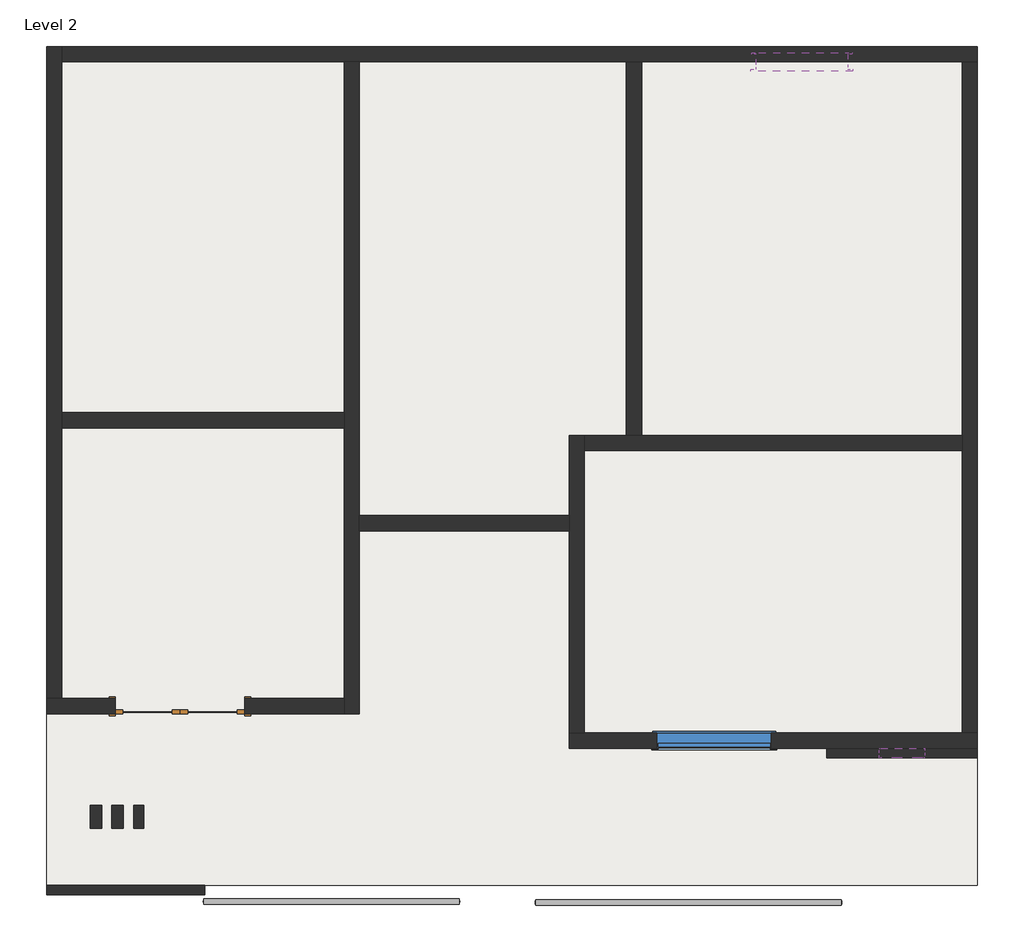
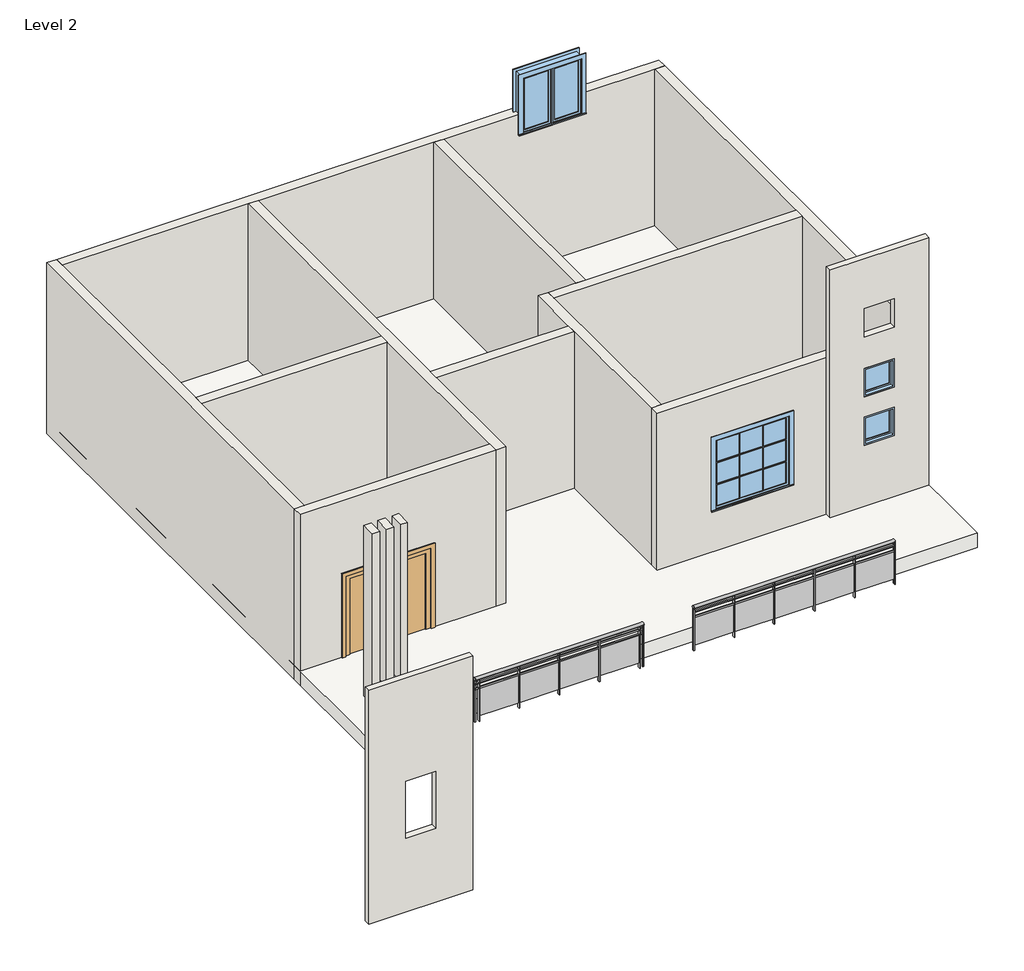
# One storey: 14 walls, 4 windows, 2 railings, 1 door, 1 roof.
"""IFC4 building model written with IfcOpenShell, lengths in millimetres."""

from ifc_helpers import new_model, si_unit, point, frame, origin, place, context, project, spatial, polyline, ellipse_curve, trimmed, outline, extrude, faceted_brep, transform, mapped, element, save
from ifc_brep_helpers import plane_surface, extruded_surface, advanced_brep
from components import door_10418eaf, walls_4_walls_4_19af3613, window_9e391526, window_0862ab64, window_d757e824

model = new_model("IFC4")

# Units and contexts
model_context = context("Model", 3, world=origin())
ifc_project = project(units=[si_unit("LENGTHUNIT", "METRE", prefix="MILLI")], contexts=[model_context])

# Site, building, storey
site = spatial("IfcSite", under=ifc_project)
building = spatial("IfcBuilding", under=site)
storey = spatial("IfcBuildingStorey", under=building, Name="Level 2", Elevation=3657.6)

# Door
placement = place(None, origin())
door_shape = door_10418eaf(model_context)
element("IfcDoor", 1, ObjectType="Door-Double-Glass : 68\" x 80\"", at=placement, inside=storey, context=model_context, shape_type="MappedRepresentation", body=[
    mapped(door_shape, transform((-13987.530251, 5267.654346, 3657.6), x_axis=(-1.0, 0.0, 0.0), y_axis=(0.0, -1.0, 0.0), z_axis=(0.0, 0.0, 1.0))),
])

# Railings
element("IfcRailing", 2, ObjectType="Glass Panel - Bottom Fill", at=placement, inside=storey, context=model_context, shape_type="SolidModel", body=[
    advanced_brep(
    [(-13671.3981295, 2699.873096, 4572.0), (-13671.3981295, 2623.673096, 4572.0), (-10267.7981295, 2699.873096, 4572.0), (-10267.7981295, 2623.673096, 4572.0)],
    [
        (0, 1, ellipse_curve(frame((-13671.3981295, 2661.773096, 4572.0), z_axis=(-1.0, 0.0, 0.0), x_axis=(0.0, -1.0, 0.0)), 38.1, 28.575)),
        (1, 0, ellipse_curve(frame((-13671.3981295, 2661.773096, 4572.0), z_axis=(-1.0, 0.0, 0.0), x_axis=(0.0, -1.0, 0.0)), 38.1, 28.575)),
        (2, 3, ellipse_curve(frame((-10267.7981295, 2661.773096, 4572.0), z_axis=(1.0, 0.0, 0.0), x_axis=(0.0, -1.0, 0.0)), 38.1, 28.575)),
        (3, 2, ellipse_curve(frame((-10267.7981295, 2661.773096, 4572.0), z_axis=(1.0, 0.0, 0.0), x_axis=(0.0, -1.0, 0.0)), 38.1, 28.575)),
        (0, 2),
        (3, 1),
    ],
    [
        plane_surface(frame((-13671.3981295, 2661.773096, 4572.0), z_axis=(-1.0, 0.0, 0.0), x_axis=(0.0, 1.0, 0.0))),
        plane_surface(frame((-10267.7981295, 2661.773096, 4572.0), z_axis=(1.0, 0.0, 0.0), x_axis=(0.0, 1.0, 0.0))),
        extruded_surface(trimmed(ellipse_curve(frame((-10267.7981295, 2661.773096, 4572.0), z_axis=(-1.0, 0.0, 0.0), x_axis=(0.0, -1.0, 0.0)), 38.1, 28.575), [point((-10267.7981295, 2699.873096, 4572.0))], [point((-10267.7981295, 2623.673096, 4572.0))], True, "CARTESIAN"), (-3403.5999999999985, 0.0, 0.0), 3403.5999999999985),
        extruded_surface(trimmed(ellipse_curve(frame((-10267.7981295, 2661.773096, 4572.0), z_axis=(-1.0, 0.0, 0.0), x_axis=(0.0, -1.0, 0.0)), 38.1, 28.575), [point((-10267.7981295, 2623.673096, 4572.0))], [point((-10267.7981295, 2699.873096, 4572.0))], True, "CARTESIAN"), (-3403.5999999999985, 0.0, 0.0), 3403.5999999999985),
    ],
    [
        (0, [[1, 2]]),
        (1, [[3, 4]]),
        (2, [[-1, 5, -4, 6]]),
        (3, [[-2, -6, -3, -5]]),
    ],
),
    extrude(outline(polyline([(-13671.3981295, 2649.073096), (-13671.3981295, 2674.473096), (-10267.7981295, 2674.473096), (-10267.7981295, 2649.073096), (-13671.3981295, 2649.073096)])), frame((0.0, 0.0, 4457.7), z_axis=(0.0, 0.0, 1.0), x_axis=(1.0, 0.0, 0.0)), (0.0, 0.0, 1.0), 25.4),
    extrude(outline(polyline([(-13671.3981295, 2649.073096), (-13671.3981295, 2674.473096), (-10267.7981295, 2674.473096), (-10267.7981295, 2649.073096), (-13671.3981295, 2649.073096)])), frame((0.0, 0.0, 4356.1), z_axis=(0.0, 0.0, 1.0), x_axis=(1.0, 0.0, 0.0)), (0.0, 0.0, 1.0), 25.4),
    extrude(outline(polyline([(-10350.3481295, 2636.373096), (-10350.3481295, 2687.173096), (-10337.6481295, 2687.173096), (-10337.6481295, 2636.373096), (-10350.3481295, 2636.373096)])), frame((0.0, 0.0, 3657.6), z_axis=(0.0, 0.0, 1.0), x_axis=(1.0, 0.0, 0.0)), (0.0, 0.0, 1.0), 885.6788223),
    extrude(outline(polyline([(-11156.7981295, 2668.308253), (-10343.9981295, 2668.308253), (-10343.9981295, 2661.958253), (-11156.7981295, 2661.958253), (-11156.7981295, 2668.308253)])), frame((0.0, 0.0, 3759.2), z_axis=(0.0, 0.0, 1.0), x_axis=(1.0, 0.0, 0.0)), (0.0, 0.0, 1.0), 596.9),
    extrude(outline(polyline([(-11163.1481295, 2636.373096), (-11163.1481295, 2687.173096), (-11150.4481295, 2687.173096), (-11150.4481295, 2636.373096), (-11163.1481295, 2636.373096)])), frame((0.0, 0.0, 3657.6), z_axis=(0.0, 0.0, 1.0), x_axis=(1.0, 0.0, 0.0)), (0.0, 0.0, 1.0), 885.6788223),
    extrude(outline(polyline([(-11969.5981295, 2668.308253), (-11156.7981295, 2668.308253), (-11156.7981295, 2661.958253), (-11969.5981295, 2661.958253), (-11969.5981295, 2668.308253)])), frame((0.0, 0.0, 3759.2), z_axis=(0.0, 0.0, 1.0), x_axis=(1.0, 0.0, 0.0)), (0.0, 0.0, 1.0), 596.9),
    extrude(outline(polyline([(-11975.9481295, 2636.373096), (-11975.9481295, 2687.173096), (-11963.2481295, 2687.173096), (-11963.2481295, 2636.373096), (-11975.9481295, 2636.373096)])), frame((0.0, 0.0, 3657.6), z_axis=(0.0, 0.0, 1.0), x_axis=(1.0, 0.0, 0.0)), (0.0, 0.0, 1.0), 885.6788223),
    extrude(outline(polyline([(-12782.3981295, 2668.308253), (-11969.5981295, 2668.308253), (-11969.5981295, 2661.958253), (-12782.3981295, 2661.958253), (-12782.3981295, 2668.308253)])), frame((0.0, 0.0, 3759.2), z_axis=(0.0, 0.0, 1.0), x_axis=(1.0, 0.0, 0.0)), (0.0, 0.0, 1.0), 596.9),
    extrude(outline(polyline([(-12788.7481295, 2636.373096), (-12788.7481295, 2687.173096), (-12776.0481295, 2687.173096), (-12776.0481295, 2636.373096), (-12788.7481295, 2636.373096)])), frame((0.0, 0.0, 3657.6), z_axis=(0.0, 0.0, 1.0), x_axis=(1.0, 0.0, 0.0)), (0.0, 0.0, 1.0), 885.6788223),
    extrude(outline(polyline([(-13595.1981295, 2668.308253), (-12782.3981295, 2668.308253), (-12782.3981295, 2661.958253), (-13595.1981295, 2661.958253), (-13595.1981295, 2668.308253)])), frame((0.0, 0.0, 3759.2), z_axis=(0.0, 0.0, 1.0), x_axis=(1.0, 0.0, 0.0)), (0.0, 0.0, 1.0), 596.9),
    extrude(outline(polyline([(-13601.5481295, 2636.373096), (-13601.5481295, 2687.173096), (-13588.8481295, 2687.173096), (-13588.8481295, 2636.373096), (-13601.5481295, 2636.373096)])), frame((0.0, 0.0, 3657.6), z_axis=(0.0, 0.0, 1.0), x_axis=(1.0, 0.0, 0.0)), (0.0, 0.0, 1.0), 885.6788223),
    extrude(outline(polyline([(-10280.4981295, 2652.248096), (-10280.4981295, 2671.298096), (-10261.4481295, 2671.298096), (-10261.4481295, 2652.248096), (-10280.4981295, 2652.248096)])), frame((0.0, 0.0, 3657.6), z_axis=(0.0, 0.0, 1.0), x_axis=(1.0, 0.0, 0.0)), (0.0, 0.0, 1.0), 885.6788223),
    extrude(outline(polyline([(-13677.7481295, 2652.248096), (-13677.7481295, 2671.298096), (-13658.6981295, 2671.298096), (-13658.6981295, 2652.248096), (-13677.7481295, 2652.248096)])), frame((0.0, 0.0, 3657.6), z_axis=(0.0, 0.0, 1.0), x_axis=(1.0, 0.0, 0.0)), (0.0, 0.0, 1.0), 885.6788223),
])
element("IfcRailing", 3, ObjectType="Glass Panel - Bottom Fill", at=placement, inside=storey, context=model_context, shape_type="SolidModel", body=[
    advanced_brep(
    [(-9251.7981295, 2687.173096, 4572.0), (-9251.7981295, 2610.973096, 4572.0), (-5183.7223535, 2687.173096, 4572.0), (-5183.7223535, 2610.973096, 4572.0)],
    [
        (0, 1, ellipse_curve(frame((-9251.7981295, 2649.073096, 4572.0), z_axis=(-1.0, 0.0, 0.0), x_axis=(0.0, -1.0, 0.0)), 38.1, 28.575)),
        (1, 0, ellipse_curve(frame((-9251.7981295, 2649.073096, 4572.0), z_axis=(-1.0, 0.0, 0.0), x_axis=(0.0, -1.0, 0.0)), 38.1, 28.575)),
        (2, 3, ellipse_curve(frame((-5183.7223535, 2649.073096, 4572.0), z_axis=(1.0, 0.0, 0.0), x_axis=(0.0, -1.0, 0.0)), 38.1, 28.575)),
        (3, 2, ellipse_curve(frame((-5183.7223535, 2649.073096, 4572.0), z_axis=(1.0, 0.0, 0.0), x_axis=(0.0, -1.0, 0.0)), 38.1, 28.575)),
        (0, 2),
        (3, 1),
    ],
    [
        plane_surface(frame((-9251.7981295, 2649.073096, 4572.0), z_axis=(-1.0, 0.0, 0.0), x_axis=(0.0, 1.0, 0.0))),
        plane_surface(frame((-5183.7223535, 2649.073096, 4572.0), z_axis=(1.0, 0.0, 0.0), x_axis=(0.0, 1.0, 0.0))),
        extruded_surface(trimmed(ellipse_curve(frame((-5183.7223535, 2649.073096, 4572.0), z_axis=(-1.0, 0.0, 0.0), x_axis=(0.0, -1.0, 0.0)), 38.1, 28.575), [point((-5183.7223535, 2687.173096, 4572.0))], [point((-5183.7223535, 2610.973096, 4572.0))], True, "CARTESIAN"), (-4068.0757760000006, 0.0, 0.0), 4068.0757760000006),
        extruded_surface(trimmed(ellipse_curve(frame((-5183.7223535, 2649.073096, 4572.0), z_axis=(-1.0, 0.0, 0.0), x_axis=(0.0, -1.0, 0.0)), 38.1, 28.575), [point((-5183.7223535, 2610.973096, 4572.0))], [point((-5183.7223535, 2687.173096, 4572.0))], True, "CARTESIAN"), (-4068.0757760000006, 0.0, 0.0), 4068.0757760000006),
    ],
    [
        (0, [[1, 2]]),
        (1, [[3, 4]]),
        (2, [[-1, 5, -4, 6]]),
        (3, [[-2, -6, -3, -5]]),
    ],
),
    extrude(outline(polyline([(-9251.7981295, 2636.373096), (-9251.7981295, 2661.773096), (-5183.7223535, 2661.773096), (-5183.7223535, 2636.373096), (-9251.7981295, 2636.373096)])), frame((0.0, 0.0, 4457.7), z_axis=(0.0, 0.0, 1.0), x_axis=(1.0, 0.0, 0.0)), (0.0, 0.0, 1.0), 25.4),
    extrude(outline(polyline([(-9251.7981295, 2636.373096), (-9251.7981295, 2661.773096), (-5183.7223535, 2661.773096), (-5183.7223535, 2636.373096), (-9251.7981295, 2636.373096)])), frame((0.0, 0.0, 4356.1), z_axis=(0.0, 0.0, 1.0), x_axis=(1.0, 0.0, 0.0)), (0.0, 0.0, 1.0), 25.4),
    extrude(outline(polyline([(-5192.1102415, 2623.673096), (-5192.1102415, 2674.473096), (-5179.4102415, 2674.473096), (-5179.4102415, 2623.673096), (-5192.1102415, 2623.673096)])), frame((0.0, 0.0, 3657.6), z_axis=(0.0, 0.0, 1.0), x_axis=(1.0, 0.0, 0.0)), (0.0, 0.0, 1.0), 885.6788223),
    extrude(outline(polyline([(-5998.5602415, 2655.608253), (-5185.7602415, 2655.608253), (-5185.7602415, 2649.258253), (-5998.5602415, 2649.258253), (-5998.5602415, 2655.608253)])), frame((0.0, 0.0, 3759.2), z_axis=(0.0, 0.0, 1.0), x_axis=(1.0, 0.0, 0.0)), (0.0, 0.0, 1.0), 596.9),
    extrude(outline(polyline([(-6004.9102415, 2623.673096), (-6004.9102415, 2674.473096), (-5992.2102415, 2674.473096), (-5992.2102415, 2623.673096), (-6004.9102415, 2623.673096)])), frame((0.0, 0.0, 3657.6), z_axis=(0.0, 0.0, 1.0), x_axis=(1.0, 0.0, 0.0)), (0.0, 0.0, 1.0), 885.6788223),
    extrude(outline(polyline([(-6811.3602415, 2655.608253), (-5998.5602415, 2655.608253), (-5998.5602415, 2649.258253), (-6811.3602415, 2649.258253), (-6811.3602415, 2655.608253)])), frame((0.0, 0.0, 3759.2), z_axis=(0.0, 0.0, 1.0), x_axis=(1.0, 0.0, 0.0)), (0.0, 0.0, 1.0), 596.9),
    extrude(outline(polyline([(-6817.7102415, 2623.673096), (-6817.7102415, 2674.473096), (-6805.0102415, 2674.473096), (-6805.0102415, 2623.673096), (-6817.7102415, 2623.673096)])), frame((0.0, 0.0, 3657.6), z_axis=(0.0, 0.0, 1.0), x_axis=(1.0, 0.0, 0.0)), (0.0, 0.0, 1.0), 885.6788223),
    extrude(outline(polyline([(-7624.1602415, 2655.608253), (-6811.3602415, 2655.608253), (-6811.3602415, 2649.258253), (-7624.1602415, 2649.258253), (-7624.1602415, 2655.608253)])), frame((0.0, 0.0, 3759.2), z_axis=(0.0, 0.0, 1.0), x_axis=(1.0, 0.0, 0.0)), (0.0, 0.0, 1.0), 596.9),
    extrude(outline(polyline([(-7630.5102415, 2623.673096), (-7630.5102415, 2674.473096), (-7617.8102415, 2674.473096), (-7617.8102415, 2623.673096), (-7630.5102415, 2623.673096)])), frame((0.0, 0.0, 3657.6), z_axis=(0.0, 0.0, 1.0), x_axis=(1.0, 0.0, 0.0)), (0.0, 0.0, 1.0), 885.6788223),
    extrude(outline(polyline([(-8436.9602415, 2655.608253), (-7624.1602415, 2655.608253), (-7624.1602415, 2649.258253), (-8436.9602415, 2649.258253), (-8436.9602415, 2655.608253)])), frame((0.0, 0.0, 3759.2), z_axis=(0.0, 0.0, 1.0), x_axis=(1.0, 0.0, 0.0)), (0.0, 0.0, 1.0), 596.9),
    extrude(outline(polyline([(-8443.3102415, 2623.673096), (-8443.3102415, 2674.473096), (-8430.6102415, 2674.473096), (-8430.6102415, 2623.673096), (-8443.3102415, 2623.673096)])), frame((0.0, 0.0, 3657.6), z_axis=(0.0, 0.0, 1.0), x_axis=(1.0, 0.0, 0.0)), (0.0, 0.0, 1.0), 885.6788223),
    extrude(outline(polyline([(-9249.7602415, 2655.608253), (-8436.9602415, 2655.608253), (-8436.9602415, 2649.258253), (-9249.7602415, 2649.258253), (-9249.7602415, 2655.608253)])), frame((0.0, 0.0, 3759.2), z_axis=(0.0, 0.0, 1.0), x_axis=(1.0, 0.0, 0.0)), (0.0, 0.0, 1.0), 596.9),
    extrude(outline(polyline([(-9256.1102415, 2623.673096), (-9256.1102415, 2674.473096), (-9243.4102415, 2674.473096), (-9243.4102415, 2623.673096), (-9256.1102415, 2623.673096)])), frame((0.0, 0.0, 3657.6), z_axis=(0.0, 0.0, 1.0), x_axis=(1.0, 0.0, 0.0)), (0.0, 0.0, 1.0), 885.6788223),
    extrude(outline(polyline([(-5196.4223535, 2639.548096), (-5196.4223535, 2658.598096), (-5177.3723535, 2658.598096), (-5177.3723535, 2639.548096), (-5196.4223535, 2639.548096)])), frame((0.0, 0.0, 3657.6), z_axis=(0.0, 0.0, 1.0), x_axis=(1.0, 0.0, 0.0)), (0.0, 0.0, 1.0), 885.6788223),
    extrude(outline(polyline([(-9258.1481295, 2639.548096), (-9258.1481295, 2658.598096), (-9239.0981295, 2658.598096), (-9239.0981295, 2639.548096), (-9258.1481295, 2639.548096)])), frame((0.0, 0.0, 3657.6), z_axis=(0.0, 0.0, 1.0), x_axis=(1.0, 0.0, 0.0)), (0.0, 0.0, 1.0), 885.6788223),
])

# Roof
element("IfcRoof", 4, ObjectType="Generic - 12\"", at=placement, inside=storey, context=model_context, shape_type="SweptSolid", body=[
    extrude(outline(polyline([(-15765.530251, 14053.673096), (-3370.330251, 14053.673096), (-3370.330251, 2877.673096), (-12723.880251, 2877.673096), (-15765.530251, 2877.673096), (-15765.530251, 14053.673096)])), frame((0.0, 0.0, 3657.6), z_axis=(0.0, 0.0, 1.0), x_axis=(1.0, 0.0, 0.0)), (0.0, 0.0, 1.0), 304.8),
])

# Walls
element("IfcWall", 5, ObjectType="Generic - 5\"", at=placement, inside=storey, context=model_context, shape_type="Brep", body=[
    faceted_brep([(-3370.330251, 4706.473096, 3657.6), (-5376.930251, 4706.473096, 3657.6), (-5376.930251, 4706.473096, 9265.7166466), (-3370.330251, 4706.473096, 9265.7166466), (-3370.330251, 4706.473096, 8534.4), (-3370.330251, 4706.473096, 7315.2), (-4068.830251, 4706.473096, 8203.7905952), (-4678.430251, 4706.473096, 8203.7905952), (-4678.430251, 4706.473096, 7594.1905952), (-4068.830251, 4706.473096, 7594.1905952), (-4068.830251, 4706.473096, 6919.2367933), (-4678.430251, 4706.473096, 6919.2367933), (-4678.430251, 4706.473096, 6309.6367933), (-4068.830251, 4706.473096, 6309.6367933), (-4068.830251, 4706.473096, 5876.6924227), (-4678.430251, 4706.473096, 5876.6924227), (-4678.430251, 4706.473096, 5267.0924227), (-4068.830251, 4706.473096, 5267.0924227), (-3370.330251, 4579.473096, 3657.6), (-3370.330251, 4579.473096, 9265.7166466), (-5376.930251, 4579.473096, 9265.7166466), (-5376.930251, 4579.473096, 8839.2), (-5376.930251, 4579.473096, 7315.2), (-5376.930251, 4579.473096, 3657.6), (-4068.830251, 4579.473096, 8203.7905952), (-4068.830251, 4579.473096, 7594.1905952), (-4678.430251, 4579.473096, 7594.1905952), (-4678.430251, 4579.473096, 8203.7905952), (-4068.830251, 4579.473096, 6919.2367933), (-4068.830251, 4579.473096, 6309.6367933), (-4678.430251, 4579.473096, 6309.6367933), (-4678.430251, 4579.473096, 6919.2367933), (-4068.830251, 4579.473096, 5876.6924227), (-4068.830251, 4579.473096, 5267.0924227), (-4678.430251, 4579.473096, 5267.0924227), (-4678.430251, 4579.473096, 5876.6924227)], [[[0, 1, 2, 3, 4, 5], [6, 7, 8, 9], [10, 11, 12, 13], [14, 15, 16, 17]], [[18, 19, 20, 21, 22, 23], [24, 25, 26, 27], [28, 29, 30, 31], [32, 33, 34, 35]], [[1, 0, 18, 23]], [[3, 2, 20, 19]], [[2, 1, 23, 22, 21, 20]], [[0, 5, 4, 3, 19, 18]], [[25, 24, 6, 9]], [[26, 25, 9, 8]], [[27, 26, 8, 7]], [[24, 27, 7, 6]], [[29, 28, 10, 13]], [[30, 29, 13, 12]], [[31, 30, 12, 11]], [[28, 31, 11, 10]], [[33, 32, 14, 17]], [[34, 33, 17, 16]], [[35, 34, 16, 15]], [[32, 35, 15, 14]]]),
])
element("IfcWall", 6, ObjectType="Generic - 5\"", at=placement, inside=storey, context=model_context, shape_type="SweptSolid", body=[
    extrude(outline(polyline([(0.0, -15765.530251), (0.0, -13657.330251), (5008.6690513, -13657.330251), (5008.6690513, -15765.530251), (0.0, -15765.530251)]), holes=[polyline([(2806.4056944, -14406.630251), (1587.2056944, -14406.630251), (1587.2056944, -15016.230251), (2806.4056944, -15016.230251), (2806.4056944, -14406.630251)])]), frame((0.0, 2750.673096, 0.0), z_axis=(0.0, 1.0, 0.0), x_axis=(0.0, 0.0, 1.0)), (0.0, 0.0, 1.0), 127.0),
])
element("IfcWall", 7, ObjectType="Generic - 8\"", at=placement, inside=storey, context=model_context, shape_type="Brep", body=[
    faceted_brep([(-3370.330251, 4909.673096, 3657.6), (-3573.530251, 4909.673096, 3657.6), (-8602.730251, 4909.673096, 3657.6), (-8805.930251, 4909.673096, 3657.6), (-8805.930251, 4909.673096, 7315.2), (-8602.730251, 4909.673096, 7315.2), (-3573.530251, 4909.673096, 7315.2), (-3370.330251, 4909.673096, 7315.2), (-7637.530251, 4909.673096, 6357.9072246), (-7637.530251, 4909.673096, 4833.9072246), (-6113.530251, 4909.673096, 4833.9072246), (-6113.530251, 4909.673096, 6357.9072246), (-3370.330251, 4706.473096, 3657.6), (-3370.330251, 4706.473096, 7315.2), (-5249.930251, 4706.473096, 7315.2), (-8805.930251, 4706.473096, 7315.2), (-8805.930251, 4706.473096, 3657.6), (-7637.530251, 4706.473096, 6357.9072246), (-6113.530251, 4706.473096, 6357.9072246), (-6113.530251, 4706.473096, 4833.9072246), (-7637.530251, 4706.473096, 4833.9072246)], [[[0, 1, 2, 3, 4, 5, 6, 7], [8, 9, 10, 11]], [[12, 13, 14, 15, 16], [17, 18, 19, 20]], [[3, 2, 1, 0, 12, 16]], [[4, 3, 16, 15]], [[0, 7, 13, 12]], [[7, 6, 5, 4, 15, 14, 13]], [[9, 8, 17, 20]], [[10, 9, 20, 19]], [[11, 10, 19, 18]], [[8, 11, 18, 17]]]),
])
element("IfcWall", 8, ObjectType="Generic - 8\"", at=placement, inside=storey, context=model_context, shape_type="Brep", body=[
    faceted_brep([(-8602.730251, 4909.673096, 3657.6), (-8602.730251, 8668.873096, 3657.6), (-8602.730251, 8872.073096, 3657.6), (-8602.730251, 8872.073096, 7315.2), (-8602.730251, 8668.873096, 7315.2), (-8602.730251, 4909.673096, 7315.2), (-8805.930251, 4909.673096, 3657.6), (-8805.930251, 4909.673096, 7315.2), (-8805.930251, 7602.073096, 7315.2), (-8805.930251, 7805.273096, 7315.2), (-8805.930251, 8872.073096, 7315.2), (-8805.930251, 8872.073096, 3657.6), (-8805.930251, 7805.273096, 3657.6), (-8805.930251, 7602.073096, 3657.6)], [[[0, 1, 2, 3, 4, 5]], [[6, 7, 8, 9, 10, 11, 12, 13]], [[2, 1, 0, 6, 13, 12, 11]], [[0, 5, 7, 6]], [[3, 2, 11, 10]], [[5, 4, 3, 10, 9, 8, 7]]]),
])
element("IfcWall", 9, ObjectType="Generic - 8\"", at=placement, inside=storey, context=model_context, shape_type="Brep", body=[
    faceted_brep([(-8602.730251, 8668.873096, 3657.6), (-3573.530251, 8668.873096, 3657.6), (-3573.530251, 8668.873096, 7315.2), (-8602.730251, 8668.873096, 7315.2), (-8602.730251, 8872.073096, 3657.6), (-8602.730251, 8872.073096, 7315.2), (-8043.930251, 8872.073096, 7315.2), (-7840.730251, 8872.073096, 7315.2), (-3573.530251, 8872.073096, 7315.2), (-3573.530251, 8872.073096, 3657.6), (-7840.730251, 8872.073096, 3657.6), (-8043.930251, 8872.073096, 3657.6)], [[[0, 1, 2, 3]], [[4, 5, 6, 7, 8, 9, 10, 11]], [[1, 0, 4, 11, 10, 9]], [[0, 3, 5, 4]], [[2, 1, 9, 8]], [[3, 2, 8, 7, 6, 5]]]),
])
element("IfcWall", 10, ObjectType="Generic - 8\"", at=placement, inside=storey, context=model_context, shape_type="Brep", body=[
    faceted_brep([(-3370.330251, 4909.673096, 3657.6), (-3370.330251, 13850.473096, 3657.6), (-3370.330251, 13850.473096, 7315.2), (-3370.330251, 4909.673096, 7315.2), (-3573.530251, 4909.673096, 3657.6), (-3573.530251, 4909.673096, 7315.2), (-3573.530251, 8668.873096, 7315.2), (-3573.530251, 8872.073096, 7315.2), (-3573.530251, 13850.473096, 7315.2), (-3573.530251, 13850.473096, 3657.6), (-3573.530251, 8872.073096, 3657.6), (-3573.530251, 8668.873096, 3657.6)], [[[0, 1, 2, 3]], [[4, 5, 6, 7, 8, 9, 10, 11]], [[1, 0, 4, 11, 10, 9]], [[0, 3, 5, 4]], [[2, 1, 9, 8]], [[3, 2, 8, 7, 6, 5]]]),
])
element("IfcWall", 11, ObjectType="Generic - 8\"", at=placement, inside=storey, context=model_context, shape_type="SweptSolid", body=[
    extrude(outline(polyline([(-11599.930251, 7805.273096), (-8805.930251, 7805.273096), (-8805.930251, 7602.073096), (-11599.930251, 7602.073096), (-11599.930251, 7805.273096)])), frame((0.0, 0.0, 3657.6), z_axis=(0.0, 0.0, 1.0), x_axis=(1.0, 0.0, 0.0)), (0.0, 0.0, 1.0), 3657.6),
])
element("IfcWall", 12, ObjectType="Generic - 8\"", at=placement, inside=storey, context=model_context, shape_type="Brep", body=[
    faceted_brep([(-11803.130251, 13850.473096, 3657.6), (-11803.130251, 9176.873096, 3657.6), (-11803.130251, 8973.673096, 3657.6), (-11803.130251, 5366.873096, 3657.6), (-11803.130251, 5163.673096, 3657.6), (-11803.130251, 5163.673096, 7315.2), (-11803.130251, 5366.873096, 7315.2), (-11803.130251, 8973.673096, 7315.2), (-11803.130251, 9176.873096, 7315.2), (-11803.130251, 13850.473096, 7315.2), (-11599.930251, 13850.473096, 3657.6), (-11599.930251, 13850.473096, 7315.2), (-11599.930251, 7805.273096, 7315.2), (-11599.930251, 7602.073096, 7315.2), (-11599.930251, 5163.673096, 7315.2), (-11599.930251, 5163.673096, 3657.6), (-11599.930251, 7602.073096, 3657.6), (-11599.930251, 7805.273096, 3657.6)], [[[0, 1, 2, 3, 4, 5, 6, 7, 8, 9]], [[10, 11, 12, 13, 14, 15, 16, 17]], [[4, 3, 2, 1, 0, 10, 17, 16, 15]], [[5, 4, 15, 14]], [[0, 9, 11, 10]], [[9, 8, 7, 6, 5, 14, 13, 12, 11]]]),
])
element("IfcWall", 13, ObjectType="Generic - 8\"", at=placement, inside=storey, context=model_context, shape_type="Brep", body=[
    faceted_brep([(-14851.130251, 5366.873096, 5689.6), (-14851.130251, 5366.873096, 3657.6), (-15562.330251, 5366.873096, 3657.6), (-15765.530251, 5366.873096, 3657.6), (-15765.530251, 5366.873096, 7315.2), (-15562.330251, 5366.873096, 7315.2), (-11803.130251, 5366.873096, 7315.2), (-11803.130251, 5366.873096, 3657.6), (-13123.930251, 5366.873096, 3657.6), (-13123.930251, 5366.873096, 5689.6), (-15765.530251, 5163.673096, 3657.6), (-14851.130251, 5163.673096, 3657.6), (-14851.130251, 5163.673096, 5689.6), (-13123.930251, 5163.673096, 5689.6), (-13123.930251, 5163.673096, 3657.6), (-11803.130251, 5163.673096, 3657.6), (-11803.130251, 5163.673096, 7315.2), (-15765.530251, 5163.673096, 7315.2)], [[[0, 1, 2, 3, 4, 5, 6, 7, 8, 9]], [[10, 11, 12, 13, 14, 15, 16, 17]], [[8, 7, 15, 14]], [[3, 2, 1, 11, 10]], [[7, 6, 16, 15]], [[4, 3, 10, 17]], [[6, 5, 4, 17, 16]], [[12, 11, 1, 0]], [[13, 12, 0, 9]], [[14, 13, 9, 8]]]),
])
element("IfcWall", 14, ObjectType="Generic - 8\"", at=placement, inside=storey, context=model_context, shape_type="Brep", body=[
    faceted_brep([(-15562.330251, 5366.873096, 3657.6), (-15562.330251, 8973.673096, 3657.6), (-15562.330251, 9176.873096, 3657.6), (-15562.330251, 13850.473096, 3657.6), (-15562.330251, 14053.673096, 3657.6), (-15562.330251, 14053.673096, 7315.2), (-15562.330251, 13850.473096, 7315.2), (-15562.330251, 9176.873096, 7315.2), (-15562.330251, 8973.673096, 7315.2), (-15562.330251, 5366.873096, 7315.2), (-15765.530251, 5366.873096, 3657.6), (-15765.530251, 5366.873096, 7315.2), (-15765.530251, 14053.673096, 7315.2), (-15765.530251, 14053.673096, 3657.6)], [[[0, 1, 2, 3, 4, 5, 6, 7, 8, 9]], [[10, 11, 12, 13]], [[4, 3, 2, 1, 0, 10, 13]], [[0, 9, 11, 10]], [[5, 4, 13, 12]], [[9, 8, 7, 6, 5, 12, 11]]]),
])
element("IfcWall", 15, ObjectType="Generic - 8\"", at=placement, inside=storey, context=model_context, shape_type="Brep", body=[
    faceted_brep([(-15562.330251, 13850.473096, 3657.6), (-11803.130251, 13850.473096, 3657.6), (-11599.930251, 13850.473096, 3657.6), (-8043.930251, 13850.473096, 3657.6), (-7840.730251, 13850.473096, 3657.6), (-3573.530251, 13850.473096, 3657.6), (-3370.330251, 13850.473096, 3657.6), (-3370.330251, 13850.473096, 7315.2), (-3573.530251, 13850.473096, 7315.2), (-5097.530251, 13850.473096, 7315.2), (-5097.530251, 13850.473096, 6949.6474745), (-6316.730251, 13850.473096, 6949.6474745), (-6316.730251, 13850.473096, 7315.2), (-7840.730251, 13850.473096, 7315.2), (-8043.930251, 13850.473096, 7315.2), (-11599.930251, 13850.473096, 7315.2), (-11803.130251, 13850.473096, 7315.2), (-15562.330251, 13850.473096, 7315.2), (-3370.330251, 14053.673096, 3657.6), (-15562.330251, 14053.673096, 3657.6), (-15562.330251, 14053.673096, 7315.2), (-6316.730251, 14053.673096, 7315.2), (-6316.730251, 14053.673096, 6949.6474745), (-5097.530251, 14053.673096, 6949.6474745), (-5097.530251, 14053.673096, 7315.2), (-3370.330251, 14053.673096, 7315.2)], [[[0, 1, 2, 3, 4, 5, 6, 7, 8, 9, 10, 11, 12, 13, 14, 15, 16, 17]], [[18, 19, 20, 21, 22, 23, 24, 25]], [[6, 5, 4, 3, 2, 1, 0, 19, 18]], [[0, 17, 20, 19]], [[7, 6, 18, 25]], [[20, 17, 16, 15, 14, 13, 12, 21]], [[7, 25, 24, 9, 8]], [[11, 22, 21, 12]], [[22, 11, 10, 23]], [[23, 10, 9, 24]]]),
])
element("IfcWall", 16, ObjectType="Generic - 8\"", at=placement, inside=storey, context=model_context, shape_type="SweptSolid", body=[
    extrude(outline(polyline([(-15562.330251, 9176.873096), (-11803.130251, 9176.873096), (-11803.130251, 8973.673096), (-15562.330251, 8973.673096), (-15562.330251, 9176.873096)])), frame((0.0, 0.0, 3657.6), z_axis=(0.0, 0.0, 1.0), x_axis=(1.0, 0.0, 0.0)), (0.0, 0.0, 1.0), 3657.6),
])
element("IfcWall", 17, ObjectType="Generic - 8\"", at=placement, inside=storey, context=model_context, shape_type="SweptSolid", body=[
    extrude(outline(polyline([(-7840.730251, 13850.473096), (-7840.730251, 8872.073096), (-8043.930251, 8872.073096), (-8043.930251, 13850.473096), (-7840.730251, 13850.473096)])), frame((0.0, 0.0, 3657.6), z_axis=(0.0, 0.0, 1.0), x_axis=(1.0, 0.0, 0.0)), (0.0, 0.0, 1.0), 3657.6),
])
walls_4_walls_4_shape = walls_4_walls_4_19af3613(model_context)
element("IfcWall", 18, ObjectType="Walls 4 : Walls 4", at=placement, inside=storey, context=model_context, shape_type="MappedRepresentation", body=[
    mapped(walls_4_walls_4_shape, transform((0.0, 0.0, 0.0), x_axis=(1.0, 0.0, 0.0), y_axis=(0.0, 1.0, 0.0), z_axis=(0.0, 0.0, 1.0))),
])

# Windows
window_shape = window_9e391526(model_context)
element("IfcWindow", 19, ObjectType="Casement 3x3 with Trim : 60\" x 60\"", at=placement, inside=storey, context=model_context, shape_type="MappedRepresentation", body=[
    mapped(window_shape, transform((-6875.530251, 4808.073096, 3919.5072246), x_axis=(-1.0, 0.0, 0.0), y_axis=(0.0, -1.0, 0.0), z_axis=(0.0, 0.0, 1.0))),
])
window_2_shape = window_0862ab64(model_context)
element("IfcWindow", 20, ObjectType="Casement Dbl with Trim.0001 : 48\" x 48\"", at=placement, inside=storey, context=model_context, shape_type="MappedRepresentation", body=[
    mapped(window_2_shape, transform((-5707.130251, 13869.523096, 6035.2474745), x_axis=(-1.0, 0.0, 0.0), y_axis=(0.0, -1.0, 0.0), z_axis=(0.0, 0.0, 1.0))),
])
window_3_shape = window_d757e824(model_context)
element("IfcWindow", 21, ObjectType="Fixed : 24\" x 24\"", at=placement, inside=storey, context=model_context, shape_type="MappedRepresentation", body=[
    mapped(window_3_shape, transform((-4335.530251, 4642.973096, 5395.2367933), x_axis=(1.0, 0.0, 0.0), y_axis=(0.0, 1.0, 0.0), z_axis=(0.0, 0.0, 1.0))),
])
element("IfcWindow", 22, ObjectType="Fixed : 24\" x 24\"", at=placement, inside=storey, context=model_context, shape_type="MappedRepresentation", body=[
    mapped(window_3_shape, transform((-4335.530251, 4642.973096, 4352.6924227), x_axis=(1.0, 0.0, 0.0), y_axis=(0.0, 1.0, 0.0), z_axis=(0.0, 0.0, 1.0))),
])

save(model, "model.ifc")

# Revit data of these elements
# Type "Door-Double-Glass : 68\" x 80\""
#   Type Mark = "8"
#   Construction Type Id = "opn-d45"
#   Assembly Code = "C1020"
#   Analytic Construction = "Wood frame, double glass door "
#   W = 2' - 10"
#   Thickness = 0' - 2"
#   Thermal Resistance (R) = 1.8150 (h·ft²·°F)/BTU
#   Swing Angle [instance default] = 90.00°
#   Heat Transfer Coefficient (U) = 0.5510 BTU/(h·ft²·°F)
#   Height = 6' - 8"
#   Bottom Rail = 0' - 4"
#   Top Rail = 0' - 4"
#   Stiles = 0' - 4"
#   Trim Projection = 0' - 1"
#   Trim Width = 0' - 3"
#   Width = 5' - 8"
#   Define Thermal Properties by = 1
#   Glazing = Glass
#   Panel Material = Wood - Birch - Solid Stained Light Low Gloss
#   Trim Material = Paint - Sienna
#   Visual Light Transmittance = 0
#   Solar Heat Gain Coefficient = 0
#   Function = (empty or 0)
#   Wall Closure = (empty or 0)
# Type "Glass Panel - Bottom Fill"
#   Assembly Code = "C2010400"
#   built-in parameter 1008612 = 0.0416667 (stored number, unit not read)
#   built-in parameter 1008611 = 0.0416667 (stored number, unit not read)
#   built-in parameter 1008609 = 0.333333 (stored number, unit not read)
#   built-in parameter 1008604 = 0.166667 (stored number, unit not read)
#   built-in parameter 1008603 = 0.166667 (stored number, unit not read)
#   Railing Height = 3' - 0"
#   built-in parameter 1008630 = 2
#   built-in parameter 1008610 = 2
#   built-in parameter 1008618 = Baluster - Square : 3/4"
# Type "Generic - 12\""
#   Assembly Code = "B1020"
#   Layers, outside or top first: 1' - 0" no material (function 1)
# Type "Generic - 5\""
#   Assembly Code = "B2010"
#   Layers, outside or top first: 0' - 5" no material (function 1)
# Type "Generic - 8\""
#   Assembly Code = "B2010"
#   Layers, outside or top first: 0' - 8" no material (function 1)
# Type "Casement 3x3 with Trim : 60\" x 60\""
#   Type Mark = "13"
#   Construction Type Id = "GSP4R"
#   Assembly Code = "B2020100"
#   Analytic Construction = "1/8 in Pilkington single glazing"
#   Visual Light Transmittance = 0.9
#   Solar Heat Gain Coefficient = 0.78
#   Heat Transfer Coefficient (U) = 0.6496 BTU/(h·ft²·°F)
#   Height = 5' - 0"
#   Default Sill Height = 3' - 0"
#   Trim Projection - Ext. = 0' - 0 1/2"
#   Trim Projection - Int. = 0' - 0 3/4"
#   Trim Width - Exterior = 0' - 3 1/2"
#   Trim Width - Interior = 0' - 3 1/2"
#   Width = 5' - 0"
#   Window Inset = 0' - 0 3/4"
#   Define Thermal Properties by = 1
#   Glass Pane Material = Glass
#   Sash Material = Sash
#   Trim Exterior Material = Trim
#   Trim Interior Material = Trim
#   Wall Closure = (empty or 0)
# Type "Casement Dbl with Trim.0001 : 48\" x 48\""
#   Type Mark = "10"
#   Construction Type Id = "GSP4R"
#   Assembly Code = "B2020100"
#   Analytic Construction = "1/8 in Pilkington single glazing"
#   Visual Light Transmittance = 0.9
#   Solar Heat Gain Coefficient = 0.78
#   Heat Transfer Coefficient (U) = 0.6496 BTU/(h·ft²·°F)
#   Height = 4' - 0"
#   Default Sill Height = 3' - 0"
#   Trim Projection - Ext. = 0' - 0 1/2"
#   Trim Projection - Int. = 0' - 0 3/4"
#   Trim Width - Exterior = 0' - 3 1/2"
#   Trim Width - Interior = 0' - 3 1/2"
#   Width = 4' - 0"
#   Window Inset = 0' - 0 3/4"
#   Define Thermal Properties by = 1
#   Glass Pane Material = Glass
#   Sash Material = Sash
#   Trim Exterior Material = Trim
#   Trim Interior Material = Trim
#   Wall Closure = (empty or 0)
# Type "Fixed : 24\" x 24\""
#   Type Mark = "3"
#   Construction Type Id = "GSP4R"
#   Assembly Code = "B2020100"
#   Analytic Construction = "1/8 in Pilkington single glazing"
#   Visual Light Transmittance = 0.9
#   Solar Heat Gain Coefficient = 0.78
#   Heat Transfer Coefficient (U) = 0.6496 BTU/(h·ft²·°F)
#   Height = 2' - 0"
#   Default Sill Height = 3' - 0"
#   Width = 2' - 0"
#   Window Inset = 0' - 0 3/4"
#   Define Thermal Properties by = 1
#   Glass Pane Material = Glass
#   Sash Material = Sash
#   Wall Closure = (empty or 0)
# Element 1 (IfcDoor, "Door-Double-Glass : 68\" x 80\"")
#   Swing Angle = 90.00°
#   Phase Created = New Construction
#   Materials on its faces: "Wood - Birch - Solid Stained Light Low Gloss", "Paint - Sienna", "Glass"
# Elements 2, 3 (IfcRailing, "Glass Panel - Bottom Fill")
#   Phase Created = New Construction
#   Materials on its faces: "Glass"
# Element 4 (IfcRoof, "Generic - 12\"")
#   built-in parameter 1001705 = 13 (stored number, unit not read)
#   built-in parameter 1001710 = 33615
#   Phase Created = New Construction
#   Materials on its faces: "Default Roof"
# Element 5 (IfcWall, "Generic - 5\"")
#   Top Offset = 6' - 4.79199"
#   Base Offset = 0' - 0"
#   wall height = 18' - 4.79199"
#   Phase Created = New Construction
#   Base Constraint = Level 2
#   Top Constraint = Level 3
#   Materials on its faces: "Default Wall"
# Element 6 (IfcWall, "Generic - 5\"")
#   built-in parameter 1001111 = -12' - 0"
#   Top Offset = -7' - 6.80831"
#   Base Offset = -12' - 0"
#   wall height = 16' - 5.19169"
#   Phase Created = New Construction
#   Base Constraint = Level 2
#   Top Constraint = Level 3
#   Materials on its faces: "Default Wall"
# Elements 7, 8, 9, 10, 11, 12, 13, 14, 15, 16, 17 (IfcWall, "Generic - 8\"")
#   Top Offset = 0' - 0"
#   Base Offset = 0' - 0"
#   Unconnected Height = 12' - 0"
#   wall height = 12' - 0"
#   Phase Created = New Construction
#   Base Constraint = Level 2
#   Materials on its faces: "Default Wall"
# Element 18 (IfcWall, "Walls 4 : Walls 4")
#   Phase Created = New Construction
#   Materials on its faces: "Default Wall"
# Element 19 (IfcWindow, "Casement 3x3 with Trim : 60\" x 60\"")
#   Mark = "6"
#   Phase Created = New Construction
#   Materials on its faces: "Sash", "Glass", "Trim"
# Element 20 (IfcWindow, "Casement Dbl with Trim.0001 : 48\" x 48\"")
#   Mark = "5"
#   Phase Created = New Construction
#   Materials on its faces: "Sash", "Trim", "Glass"
# Element 21 (IfcWindow, "Fixed : 24\" x 24\"")
#   Mark = "2"
#   Phase Created = New Construction
#   Materials on its faces: "Sash", "Glass"
# Element 22 (IfcWindow, "Fixed : 24\" x 24\"")
#   Mark = "3"
#   Phase Created = New Construction
#   Materials on its faces: "Sash", "Glass"
# Materials
#   "Glass": class "Glass", colour RGB 0 128 192, transparency 0.75, Description = "Soda Lime Glass", Cost = 0
#   "Wood - Birch - Solid Stained Light Low Gloss": class "Wood", colour RGB 210 159 95, transparency 0, Cost = 0
#   "Paint - Sienna": colour RGB 118 70 51, transparency 0, Cost = 0
#   "Sash": class "Wood", colour RGB 224 178 126, transparency 0
#   "Trim": class "Wood", colour RGB 224 178 126, transparency 0
#   "Default Roof": colour RGB 88 101 114, transparency 0
#   "Default Wall": colour RGB 128 128 128, transparency 0
